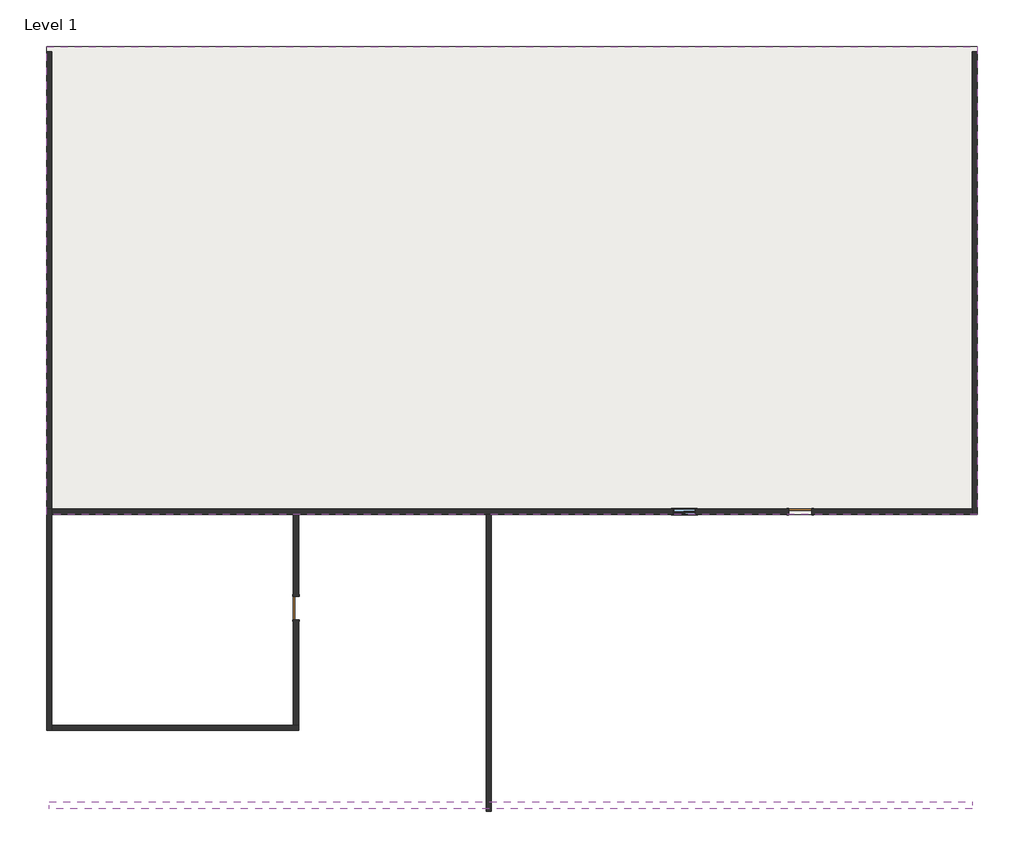
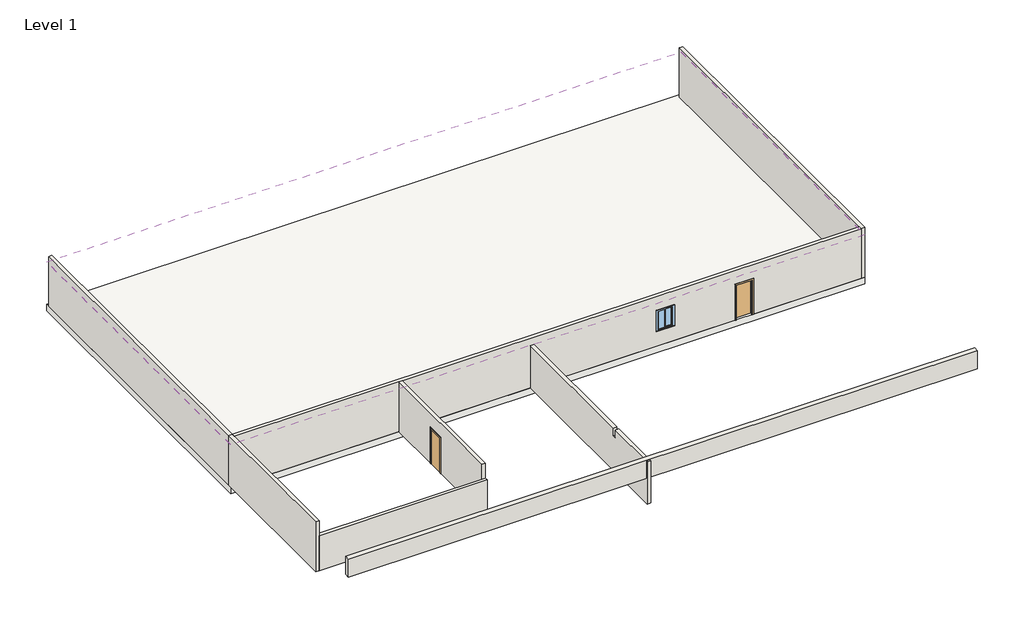
# One storey: 8 walls, 2 doors, 1 covering, 1 slab, 1 window.
"""IFC4 building model written with IfcOpenShell, lengths in millimetres."""

from ifc_helpers import new_model, si_unit, frame, origin, place, context, project, spatial, polyline, outline, extrude, faceted_brep, transform, mapped, element, save
from components import m_single_flush_0915_x_2134mm_727434cd, m_single_flush_0915_x_2134mm_6a9e8738, walls_4_walls_4_28ce44a6, window_242facca

model = new_model("IFC4")

# Units and contexts
model_context = context("Model", 3, world=origin())
ifc_project = project(units=[si_unit("LENGTHUNIT", "METRE", prefix="MILLI")], contexts=[model_context])

# Site, building, storey
site = spatial("IfcSite", under=ifc_project)
building = spatial("IfcBuilding", under=site)
storey = spatial("IfcBuildingStorey", under=building, Name="Level 1", Elevation=3048.0)

# Covering
placement = place(None, origin())
element("IfcCovering", 1, ObjectType="600 x 1200mm grid", at=placement, inside=storey, context=model_context, shape_type="SweptSolid", body=[
    extrude(outline(polyline([(17863.6339443, 17486.9935124), (17863.6339443, -1001.0064876), (-18912.3660557, -1001.0064876), (-18912.3660557, 17486.9935124), (17863.6339443, 17486.9935124)])), frame((0.0, 0.0, 5648.0), z_axis=(0.0, 0.0, 1.0), x_axis=(1.0, 0.0, 0.0)), (0.0, 0.0, 1.0), 52.0),
])

# Doors
m_single_flush_0915_x_2134mm_shape = m_single_flush_0915_x_2134mm_727434cd(model_context)
element("IfcDoor", 2, ObjectType="M_Single-Flush : 0915 x 2134mm", at=placement, inside=storey, context=model_context, shape_type="MappedRepresentation", body=[
    mapped(m_single_flush_0915_x_2134mm_shape, transform((-9058.7660557, -4711.0064876, 3048.0), x_axis=(0.0, -1.0, 0.0), y_axis=(1.0, 0.0, 0.0), z_axis=(0.0, 0.0, 1.0))),
])
m_single_flush_0915_x_2134mm_2_shape = m_single_flush_0915_x_2134mm_6a9e8738(model_context)
element("IfcDoor", 3, ObjectType="M_Single-Flush : 0915 x 2134mm", at=placement, inside=storey, context=model_context, shape_type="MappedRepresentation", body=[
    mapped(m_single_flush_0915_x_2134mm_2_shape, transform((10858.0339443, -901.0064876, 3048.0), x_axis=(1.0, 0.0, 0.0), y_axis=(0.0, 1.0, 0.0), z_axis=(0.0, 0.0, 1.0))),
])

# Slab
element("IfcSlab", 4, ObjectType="Generic Floor - 400mm", at=placement, inside=storey, context=model_context, shape_type="SweptSolid", body=[
    extrude(outline(polyline([(17863.6339443, 17486.9935124), (17863.6339443, -1001.0064876), (-18912.3660557, -1001.0064876), (-18912.3660557, 17486.9935124), (17863.6339443, 17486.9935124)])), frame((0.0, 0.0, 2648.0), z_axis=(0.0, 0.0, 1.0), x_axis=(1.0, 0.0, 0.0)), (0.0, 0.0, 1.0), 400.0),
])

# Walls
element("IfcWall", 5, ObjectType="Generic - 9\"", at=placement, inside=storey, context=model_context, shape_type="Brep", body=[
    faceted_brep([(-18712.3660557, -9535.4064876, 6096.0), (-18712.3660557, -9535.4064876, 5182.0), (-18712.3660557, -9535.4064876, 3048.0), (-18712.3660557, -9335.4064876, 3048.0), (-18712.3660557, -1001.0064876, 3048.0), (-18712.3660557, -801.0064876, 3048.0), (-18712.3660557, -801.0064876, 6096.0), (-18712.3660557, -901.0064876, 6096.0), (-18712.3660557, -1001.0064876, 6096.0), (-18712.3660557, -9335.4064876, 6096.0), (-18912.3660557, -9535.4064876, 3048.0), (-18912.3660557, -9535.4064876, 6096.0), (-18912.3660557, -801.0064876, 6096.0), (-18912.3660557, -801.0064876, 3048.0)], [[[0, 1, 2, 3, 4, 5, 6, 7, 8, 9]], [[10, 11, 12, 13]], [[5, 4, 3, 2, 10, 13]], [[0, 9, 8, 7, 6, 12, 11]], [[0, 11, 10, 2, 1]], [[5, 13, 12, 6]]]),
])
element("IfcWall", 6, ObjectType="Generic - 9\"", at=placement, inside=storey, context=model_context, shape_type="Brep", body=[
    faceted_brep([(-8958.7660557, -9335.4064876, 3048.0), (-9158.7660557, -9335.4064876, 3048.0), (-18712.3660557, -9335.4064876, 3048.0), (-18712.3660557, -9335.4064876, 5182.0), (-8958.7660557, -9335.4064876, 5182.0), (-8958.7660557, -9535.4064876, 3048.0), (-8958.7660557, -9535.4064876, 5182.0), (-18712.3660557, -9535.4064876, 5182.0), (-18712.3660557, -9535.4064876, 3048.0)], [[[0, 1, 2, 3, 4]], [[5, 6, 7, 8]], [[2, 1, 0, 5, 8]], [[4, 3, 7, 6]], [[0, 4, 6, 5]], [[3, 2, 8, 7]]]),
])
element("IfcWall", 7, ObjectType="Generic - 9\"", at=placement, inside=storey, context=model_context, shape_type="Brep", body=[
    faceted_brep([(-9158.7660557, -5168.5064876, 5182.0), (-9158.7660557, -5168.5064876, 3048.0), (-9158.7660557, -9335.4064876, 3048.0), (-9158.7660557, -9335.4064876, 6096.0), (-9158.7660557, -1001.0064876, 6096.0), (-9158.7660557, -1001.0064876, 3048.0), (-9158.7660557, -4253.5064876, 3048.0), (-9158.7660557, -4253.5064876, 5182.0), (-8958.7660557, -9335.4064876, 3048.0), (-8958.7660557, -5168.5064876, 3048.0), (-8958.7660557, -5168.5064876, 5182.0), (-8958.7660557, -4253.5064876, 5182.0), (-8958.7660557, -4253.5064876, 3048.0), (-8958.7660557, -1001.0064876, 3048.0), (-8958.7660557, -1001.0064876, 6096.0), (-8958.7660557, -9335.4064876, 6096.0), (-8958.7660557, -9335.4064876, 5182.0)], [[[0, 1, 2, 3, 4, 5, 6, 7]], [[8, 9, 10, 11, 12, 13, 14, 15, 16]], [[6, 5, 13, 12]], [[2, 1, 9, 8]], [[4, 3, 15, 14]], [[3, 2, 8, 16, 15]], [[10, 9, 1, 0]], [[11, 10, 0, 7]], [[12, 11, 7, 6]], [[4, 14, 13, 5]]]),
])
element("IfcWall", 8, ObjectType="Generic - 9\"", at=placement, inside=storey, context=model_context, shape_type="Brep", body=[
    faceted_brep([(11315.5339443, -1001.0064876, 5182.0), (11315.5339443, -1001.0064876, 3048.0), (17663.6339443, -1001.0064876, 3048.0), (17663.6339443, -1001.0064876, 6096.0), (-8958.7660557, -1001.0064876, 6096.0), (-9158.7660557, -1001.0064876, 6096.0), (-18712.3660557, -1001.0064876, 6096.0), (-18712.3660557, -1001.0064876, 3048.0), (-9158.7660557, -1001.0064876, 3048.0), (-8958.7660557, -1001.0064876, 3048.0), (-1538.7660557, -1001.0064876, 3048.0), (-1338.7660557, -1001.0064876, 3048.0), (10400.5339443, -1001.0064876, 3048.0), (10400.5339443, -1001.0064876, 5182.0), (5828.8339443, -1001.0064876, 5181.6), (6743.2339443, -1001.0064876, 5181.6), (6743.2339443, -1001.0064876, 3962.4), (5828.8339443, -1001.0064876, 3962.4), (17663.6339443, -801.0064876, 3048.0), (11315.5339443, -801.0064876, 3048.0), (11315.5339443, -801.0064876, 5182.0), (10400.5339443, -801.0064876, 5182.0), (10400.5339443, -801.0064876, 3048.0), (-18712.3660557, -801.0064876, 3048.0), (-18712.3660557, -801.0064876, 6096.0), (17663.6339443, -801.0064876, 6096.0), (5828.8339443, -801.0064876, 5181.6), (5828.8339443, -801.0064876, 3962.4), (6743.2339443, -801.0064876, 3962.4), (6743.2339443, -801.0064876, 5181.6)], [[[0, 1, 2, 3, 4, 5, 6, 7, 8, 9, 10, 11, 12, 13], [14, 15, 16, 17]], [[18, 19, 20, 21, 22, 23, 24, 25], [26, 27, 28, 29]], [[2, 1, 19, 18]], [[12, 11, 10, 9, 8, 7, 23, 22]], [[6, 5, 4, 3, 25, 24]], [[3, 2, 18, 25]], [[20, 19, 1, 0]], [[21, 20, 0, 13]], [[22, 21, 13, 12]], [[27, 26, 14, 17]], [[28, 27, 17, 16]], [[29, 28, 16, 15]], [[26, 29, 15, 14]], [[6, 24, 23, 7]]]),
])
element("IfcWall", 9, ObjectType="Generic - 9\"", at=placement, inside=storey, context=model_context, shape_type="Brep", body=[
    faceted_brep([(-18912.3660557, 17286.9935124, 3048.0), (-18912.3660557, -801.0064876, 3048.0), (-18912.3660557, -801.0064876, 6096.0), (-18912.3660557, 17286.9935124, 6096.0), (-18912.3660557, 17286.9935124, 5700.0), (-18712.3660557, 17286.9935124, 3048.0), (-18712.3660557, 17286.9935124, 6096.0), (-18712.3660557, -701.0064876, 6096.0), (-18712.3660557, -801.0064876, 6096.0), (-18712.3660557, -801.0064876, 3048.0)], [[[0, 1, 2, 3, 4]], [[5, 6, 7, 8, 9]], [[1, 0, 5, 9]], [[3, 2, 8, 7, 6]], [[1, 9, 8, 2]], [[0, 4, 3, 6, 5]]]),
])
element("IfcWall", 10, ObjectType="Generic - 9\"", at=placement, inside=storey, context=model_context, shape_type="Brep", body=[
    faceted_brep([(17863.6339443, -1001.0064876, 3048.0), (17863.6339443, 17286.9935124, 3048.0), (17863.6339443, 17286.9935124, 5700.0), (17863.6339443, 17286.9935124, 6096.0), (17863.6339443, -1001.0064876, 6096.0), (17663.6339443, -1001.0064876, 3048.0), (17663.6339443, -1001.0064876, 6096.0), (17663.6339443, -801.0064876, 6096.0), (17663.6339443, 17286.9935124, 6096.0), (17663.6339443, 17286.9935124, 3048.0), (17663.6339443, -801.0064876, 3048.0)], [[[0, 1, 2, 3, 4]], [[5, 6, 7, 8, 9, 10]], [[1, 0, 5, 10, 9]], [[4, 3, 8, 7, 6]], [[0, 4, 6, 5]], [[3, 2, 1, 9, 8]]]),
])
element("IfcWall", 11, ObjectType="Generic - 9\"", at=placement, inside=storey, context=model_context, shape_type="SweptSolid", body=[
    extrude(outline(polyline([(-1001.0064876, 3048.0), (-12737.8437646, 3048.0), (-12737.8437646, 5648.0), (-9535.4064876, 5648.0), (-9535.4064876, 5182.0), (-9335.4064876, 5182.0), (-9335.4064876, 5648.0), (-1001.0064876, 5648.0), (-1001.0064876, 3048.0)])), frame((-1538.7660557, 0.0, 0.0), z_axis=(1.0, 0.0, 0.0), x_axis=(0.0, 1.0, 0.0)), (0.0, 0.0, 1.0), 200.0),
])
walls_4_walls_4_shape = walls_4_walls_4_28ce44a6(model_context)
element("IfcWall", 12, ObjectType="Walls 4 : Walls 4", at=placement, inside=storey, context=model_context, shape_type="MappedRepresentation", body=[
    mapped(walls_4_walls_4_shape, transform((0.0, 0.0, 0.0), x_axis=(1.0, 0.0, 0.0), y_axis=(0.0, 1.0, 0.0), z_axis=(0.0, 0.0, 1.0))),
])

# Window
window_shape = window_242facca(model_context)
element("IfcWindow", 13, ObjectType="Slider with Trim : 36\" x 48\"", at=placement, inside=storey, context=model_context, shape_type="MappedRepresentation", body=[
    mapped(window_shape, transform((6286.0339443, -901.0064876, 3048.0), x_axis=(-1.0, 0.0, 0.0), y_axis=(0.0, -1.0, 0.0), z_axis=(0.0, 0.0, 1.0))),
])

save(model, "model.ifc")

# Revit data of these elements
# Type "600 x 1200mm grid"
#   built-in parameter 1002203 = 1 (stored number, unit not read)
#   built-in parameter 1002202 = 1 (stored number, unit not read)
#   Layers, outside or top first: 36 mm "Default" (function 1); 16 mm "Ceiling Tile 600 x 1200" (function 5)
# Type "M_Single-Flush : 0915 x 2134mm"
#   Type Mark = "15"
#   Thickness = 51 mm
#   Height = 2134 mm
#   Trim Projection Ext = 25 mm
#   Trim Projection Int = 25 mm
#   Trim Width = 76 mm
#   Width = 915 mm
#   Door Material = Door - Panel
#   Frame Material = Door - Frame
#   Function = (empty or 0)
#   Wall Closure = (empty or 0)
# Type "Generic Floor - 400mm"
#   Function = 0
#   Layers, outside or top first: 400 mm no material (function 1)
# Type "Generic - 9\""
#   Layers, outside or top first: 200 mm no material (function 1)
# Type "Slider with Trim : 36\" x 48\""
#   Type Mark = "19"
#   Construction Type Id = "GSP4R"
#   Assembly Code = "B2020100"
#   Analytic Construction = "1/8 in Pilkington single glazing"
#   Visual Light Transmittance = 0.9
#   Solar Heat Gain Coefficient = 0.78
#   Heat Transfer Coefficient (U) = 3.6886 W/(m²·K)
#   Height = 1219.2 mm
#   Default Sill Height = 914.4 mm
#   Trim Projection - Ext. = 19.05 mm
#   Trim Projection - Int. = 19.05 mm
#   Trim Width - Exterior = 88.9 mm
#   Trim Width - Interior = 88.9 mm
#   Width = 914.4 mm
#   Window Inset = 19.05 mm
#   Define Thermal Properties by = 1
#   Glass Pane Material = Glass
#   Sash Material = Sash
#   Trim Exterior Material = Trim
#   Trim Interior Material = Trim
#   Wall Closure = (empty or 0)
# Element 1 (IfcCovering, "600 x 1200mm grid")
#   Height Offset From Level = 2600 mm
#   Phase Created = New Construction
#   Materials on its faces: "Ceiling Tile 600 x 1200", "Default"
# Elements 2, 3 (IfcDoor, "M_Single-Flush : 0915 x 2134mm")
#   Phase Created = New Construction
#   Materials on its faces: "Door - Frame", "Door - Panel"
# Element 4 (IfcSlab, "Generic Floor - 400mm")
#   Height Offset From Level = 0 mm
#   Phase Created = New Construction
#   Materials on its faces: "Default Roof"
# Elements 5, 7, 8, 9, 10 (IfcWall, "Generic - 9\"")
#   Top Offset = 0 mm
#   Base Offset = 0 mm
#   Unconnected Height = 3048 mm
#   wall height = 3048 mm
#   Phase Created = New Construction
#   Base Constraint = Level 1
#   Materials on its faces: "Default Wall"
# Element 6 (IfcWall, "Generic - 9\"")
#   Top Offset = 0 mm
#   Base Offset = 0 mm
#   Unconnected Height = 2134 mm
#   wall height = 2134 mm
#   Phase Created = New Construction
#   Base Constraint = Level 1
#   Materials on its faces: "Default Wall"
# Element 11 (IfcWall, "Generic - 9\"")
#   Top Offset = 0 mm
#   Base Offset = 0 mm
#   Unconnected Height = 2600 mm
#   wall height = 2600 mm
#   Phase Created = New Construction
#   Base Constraint = Level 1
#   Materials on its faces: "Default Wall"
# Element 12 (IfcWall, "Walls 4 : Walls 4")
#   Phase Created = New Construction
#   Materials on its faces: "Default Wall"
# Element 13 (IfcWindow, "Slider with Trim : 36\" x 48\"")
#   Mark = "9"
#   Phase Created = New Construction
#   Materials on its faces: "Sash", "Trim", "Glass"
# Materials
#   "Default": colour RGB 80 80 80, transparency 0
#   "Ceiling Tile 600 x 1200": class "Generic", colour RGB 179 178 175, transparency 0, Description = "Acoustic ceiling tile", Cost = 0
#   "Door - Panel": class "Wood", colour RGB 114 82 51, transparency 0
#   "Door - Frame": colour RGB 153 76 43, transparency 0
#   "Glass": class "Glass", colour RGB 218 227 224, transparency 0.85, Description = "Soda Lime Glass", Cost = 0
#   "Sash": class "Wood", colour RGB 136 99 55, transparency 0
#   "Trim": class "Wood", colour RGB 224 178 126, transparency 0
#   "Default Roof": colour RGB 80 80 80, transparency 0
#   "Default Wall": colour RGB 80 80 80, transparency 0
